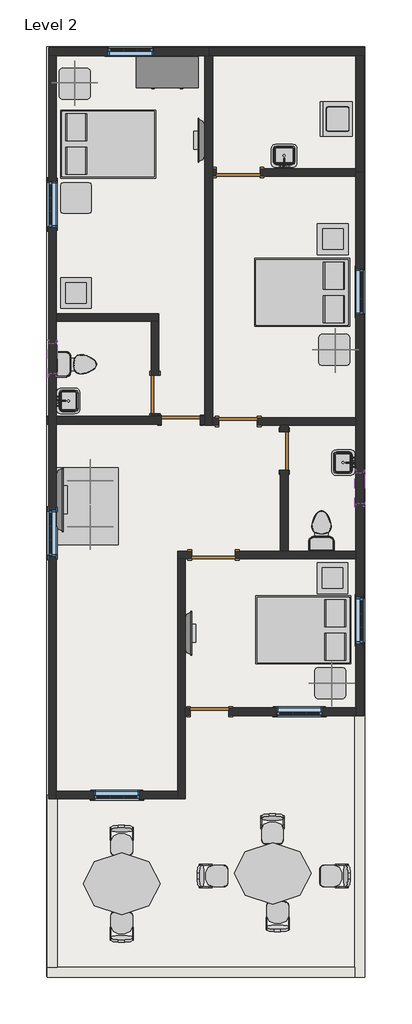
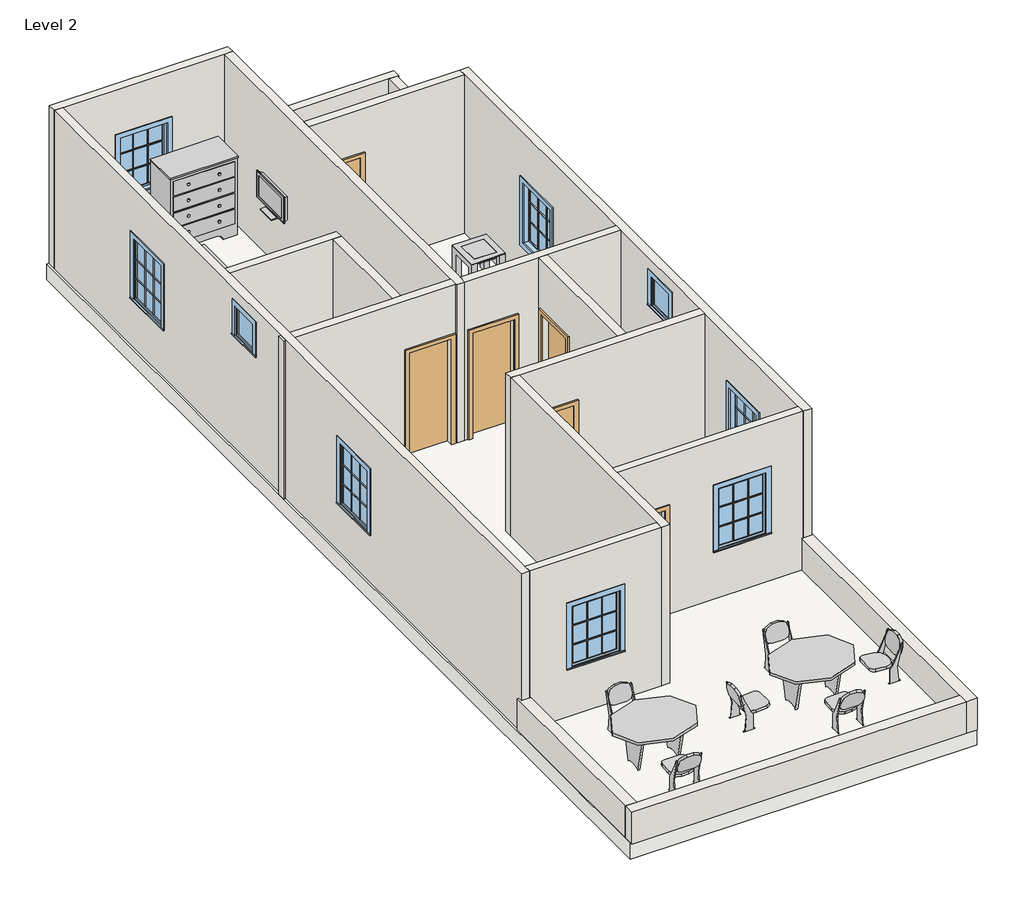
# One storey, incomplete: 23 furniture elements, 19 walls, 9 windows, 7 doors, 7 flow terminals, 5 geographic elements, 1 proxy, 1 slab.
# Revit data of these elements (continued)
# Element 28 (IfcFurniture, "TV - Flat Screen : 50\"") (continued)
#   Materials on its faces: "TV - Black", "TV - Glass", "TV - Screen"
# Elements 29, 30, 31 (IfcFurniture, "Table-Coffee : 24\" x 24\" x 24\"")
#   Phase Created = New Construction
#   Materials on its faces: "Glass - Clear, Grey"
# Elements 32, 33 (IfcFurniture, "Table-Ellipse : 60\" x 48\"")
#   Phase Created = New Construction
#   Materials on its faces: "Birch"
# Elements 34, 35, 36, 37 (IfcFurniture, "Table-End : 24\" x 24\"")
#   Phase Created = New Construction
#   Materials on its faces: "Laminate, Ivory, Matte", "Birch"
# Element 38 (IfcFurniture, "Table-Rectangular : 60\" x 48\"")
#   Phase Created = New Construction
#   Materials on its faces: "Birch"
# Elements 39, 40, 41, 42, 43 (IfcGeographicElement, "RPC Plant - Tropical : Agave - 1.5'")
#   Phase Created = New Construction
# Element 44 (IfcSlab, "Generic - 12\" 2")
#   Height Offset From Level = 0' - 0"
#   Phase Created = New Construction
#   Materials on its faces: "Brick, Common"
# Elements 45, 46, 47 (IfcWall, "Generic - 2'")
#   Top Offset = 0' - 0"
#   Base Offset = 0' - 0"
#   Unconnected Height = 2' - 0"
#   wall height = 2' - 0"
#   Phase Created = New Construction
#   Base Constraint = Level 2
#   Materials on its faces: "Birch"
# Elements 48, 50, 51, 52, 53, 54, 55, 56, 57, 58, 59, 60, 61, 63 (IfcWall, "Generic - 6'")
#   Top Offset = 0' - 0"
#   Base Offset = 0' - 0"
#   Unconnected Height = 10' - 0"
#   wall height = 10' - 0"
#   Phase Created = New Construction
#   Base Constraint = Level 2
#   Materials on its faces: "Brick, Common"
# Elements 49, 62 (IfcWall, "Generic - 6'")
#   Top Offset = 0' - 0"
#   Base Offset = 0' - 0"
#   Unconnected Height = 5' - 0"
#   wall height = 5' - 0"
#   Phase Created = New Construction
#   Base Constraint = Level 2
#   Materials on its faces: "Brick, Common"
# Element 64 (IfcWindow, "Casement 3x3 with Trim : 36\" x 48\"")
#   Mark = "7"
#   Phase Created = New Construction
#   Materials on its faces: "Sash", "Glass", "Trim"
# Element 65 (IfcWindow, "Casement 3x3 with Trim : 36\" x 48\"")
#   Mark = "8"
#   Phase Created = New Construction
#   Materials on its faces: "Sash", "Glass", "Trim"
# Element 66 (IfcWindow, "Casement 3x3 with Trim : 36\" x 48\"")
#   Mark = "9"
#   Phase Created = New Construction
#   Materials on its faces: "Sash", "Glass", "Trim"
# Element 67 (IfcWindow, "Casement 3x3 with Trim : 36\" x 48\"")
#   Mark = "10"
#   Phase Created = New Construction
#   Materials on its faces: "Sash", "Glass", "Trim"
# Element 68 (IfcWindow, "Casement 3x3 with Trim : 36\" x 48\"")
#   Mark = "11"
#   Phase Created = New Construction
#   Materials on its faces: "Sash", "Glass", "Trim"
# Element 69 (IfcWindow, "Casement 3x3 with Trim : 36\" x 48\"")
#   Mark = "12"
#   Phase Created = New Construction
#   Materials on its faces: "Sash", "Glass", "Trim"
# Element 70 (IfcWindow, "Casement 3x3 with Trim : 36\" x 48\"")
#   Mark = "13"
#   Phase Created = New Construction
#   Materials on its faces: "Sash", "Glass", "Trim"
# Element 71 (IfcWindow, "Transom with Trim : 24\" x 24\"")
#   Mark = "14"
#   Phase Created = New Construction
#   Materials on its faces: "Sash", "Trim", "Glass"
# Element 72 (IfcWindow, "Transom with Trim : 24\" x 24\"")
#   Mark = "15"
#   Phase Created = New Construction
#   Materials on its faces: "Sash", "Trim", "Glass"
# Materials
#   "Steel, Paint Finish, Ivory, Matte": class "Metal", colour RGB 247 247 239, transparency 0, Description = "Steel, paint finish, ivory, matte", Cost = 0
#   "Door - Panel": class "Wood", colour RGB 210 159 95, transparency 0
#   "Door - Frame": colour RGB 118 70 51, transparency 0
#   "Porcelain, Linen": class "Ceramic", colour RGB 249 239 230, transparency 0, Description = "Porcelain, linen", Cost = 0
#   "Steel, Polished": class "Metal", colour RGB 57 57 57, transparency 0, Description = "Polished steel", Cost = 0
#   "Laminate, Linen, Matte": class "Plastic", colour RGB 249 239 230, transparency 0, Description = "Plastic Laminate - Linen, Matte", Cost = 0
#   "Birch": class "Wood", colour RGB 224 178 126, transparency 0, Description = "Betula Alleghaniensis", Cost = 0
#   "Linen, White": class "Textile", colour RGB 247 247 239, transparency 0, Description = "Linen, white", Cost = 0
#   "Laminate - Ivory, Glossy": colour RGB 247 247 239, transparency 0
#   "Laminate, Ivory, Matte": class "Plastic", colour RGB 247 247 239, transparency 0, Description = "Plastic Laminate - Ivory, Matte", Cost = 0
#   "Cherry": class "Wood", colour RGB 226 177 128, transparency 0, Description = "Prunus Serotina", Cost = 0
#   "Linen, Beige": class "Textile", colour RGB 249 239 230, transparency 0, Description = "Linen, beige", Cost = 0
#   "Steel, Paint Finish, Dark Gray, Matte": class "Metal", colour RGB 0 0 0, transparency 0, Description = "Steel, paint finish, dark gray, matte", Cost = 0
#   "Brick, Common": class "Masonry", colour RGB 170 98 104, transparency 0, Description = "Common brick", Cost = 0
#   "Glass": class "Glass", colour RGB 0 128 192, transparency 0.75, Description = "Soda Lime Glass", Cost = 0
#   "Sash": class "Wood", colour RGB 224 178 126, transparency 0
#   "Trim": class "Wood", colour RGB 224 178 126, transparency 0
#   "TV - Black": colour RGB 49 49 49, transparency 0
#   "TV - Glass": colour RGB 157 157 157, transparency 0.9
#   "TV - Screen": colour RGB 0 0 0, transparency 0
#   "Glass - Clear, Grey": class "Glass", colour RGB 252 255 255, transparency 0.64
# Room at (-1256.493, 9199.452) mm, phase "New Construction", upper level "Level 2", upper offset 10' - 0", lower offset 0' - 0"
#   Number = "6"
#   Name = "BEDROOM"
# Room at (1702.209, 11570.611) mm, phase "New Construction", upper level "Level 2", upper offset 10' - 0", lower offset 0' - 0"
#   Number = "7"
# Room at (1702.209, 7937.297) mm, phase "New Construction", upper level "Level 2", upper offset 10' - 0", lower offset 0' - 0"
#   Number = "8"
#   Name = "BEDROOM"
# Room at (-1711.114, 6411.908) mm, phase "New Construction", upper level "Level 2", upper offset 10' - 0", lower offset 0' - 0"
#   Number = "9"
#   Name = "TOILET"
# Room at (2422.354, 3843.837) mm, phase "New Construction", upper level "Level 2", upper offset 10' - 0", lower offset 0' - 0"
#   Number = "10"
#   Name = "TOILET"
# Room at (-1079.437, 3994.584) mm, phase "New Construction", upper level "Level 2", upper offset 10' - 0", lower offset 0' - 0"
#   Number = "11"
#   Name = "LOBBY"
# Room at (1702.209, 1385.307) mm, phase "New Construction", upper level "Level 2", upper offset 10' - 0", lower offset 0' - 0"
#   Number = "12"
#   Name = "BEDROOM"
# Room at (0, -2993.9) mm, phase "New Construction", upper level "Level 2", upper offset 10' - 0", lower offset 0' - 0"
#   Number = "13"
#   Name = "LAWN/BALCONY"
